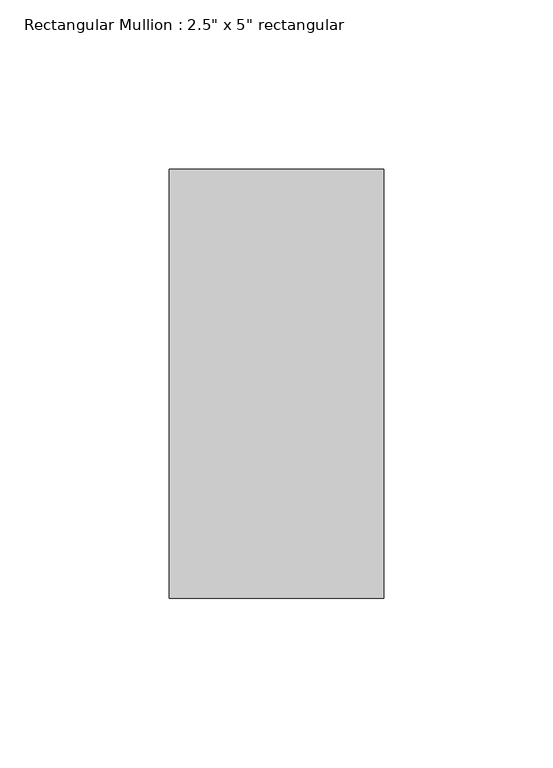
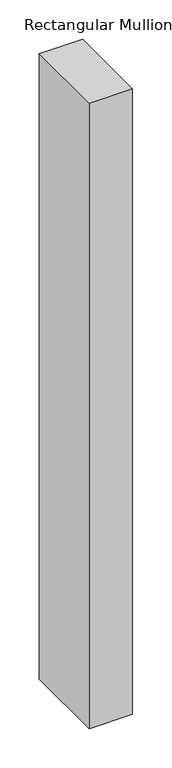
"""IFC4 building model written with IfcOpenShell, lengths in millimetres: member geometry."""

from ifc_helpers import new_model, si_unit, frame, origin, place, context, project, spatial, polyline, outline, extrude, source, transform, mapped, element, save


def member_f03bb510(model_context):
    return source(origin(), model_context, "Body", "SweptSolid", [
        extrude(outline(polyline([(0.0, 63.5), (0.0, -63.5), (-63.5, -63.5), (-63.5, 63.5), (0.0, 63.5)])), frame((0.0, 0.0, -971.5500001), z_axis=(0.0, 0.0, 1.0), x_axis=(1.0, 0.0, 0.0)), (0.0, 0.0, 1.0), 971.5500001),
    ])


if __name__ == "__main__":
    model = new_model("IFC4")
    model_context = context("Model", 3, world=origin())
    ifc_project = project(units=[si_unit("LENGTHUNIT", "METRE", prefix="MILLI")], contexts=[model_context])
    site = spatial("IfcSite", under=ifc_project)
    building = spatial("IfcBuilding", under=site)
    placement = place(None, origin())
    member_shape = member_f03bb510(model_context)
    element("IfcMember", 1, ObjectType="Rectangular Mullion : 2.5\" x 5\" rectangular", at=placement, inside=building, context=model_context, shape_type="MappedRepresentation", body=[
        mapped(member_shape, transform((0.0, 0.0, 0.0), x_axis=(1.0, 0.0, 0.0), y_axis=(0.0, 1.0, 0.0), z_axis=(0.0, 0.0, 1.0))),
    ])
    save(model, "model.ifc")

# Revit data of these elements
# Type "Rectangular Mullion : 2.5\" x 5\" rectangular"
#   built-in parameter 1007304 = 0.416667 (stored number, unit not read)
#   built-in parameter 1007301 = 0.104167 (stored number, unit not read)
#   built-in parameter 1007300 = 0.104167 (stored number, unit not read)
# Element 1 (IfcMember, "Rectangular Mullion : 2.5\" x 5\" rectangular")
#   Materials on its faces: "Aluminum"
# Materials
#   "Aluminum": class "Metal", colour RGB 247 247 247, transparency 0, Description = "Aluminum 6061", Cost = 0
